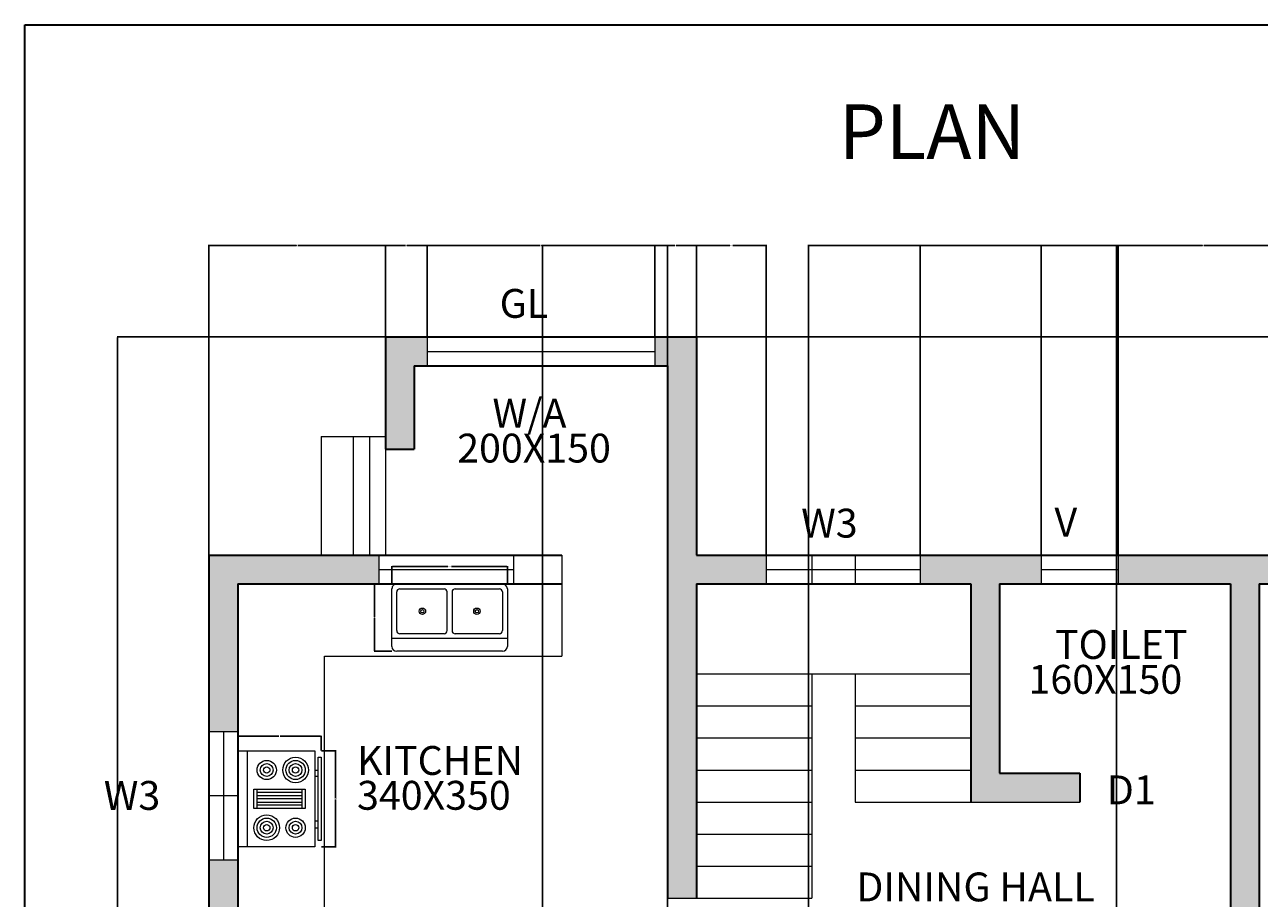
# Model space of a CAD drawing. Units: inches. Extents: x 1332 to 3175, y 1481 to 2088.
# Tile 3 of 5: x 1332 to 1717, y 1816 to 2088. Entities that reach past the tile are written whole.
import ezdxf

# ---------------------------------------------------------------- set-up
doc = ezdxf.new("R2010")
doc.units = ezdxf.units.IN
for name, color, linetype, lineweight in [('A-ANNO-DIMS', 2, 'Continuous', 18), ('A-ANNO-TEXT', 7, 'Continuous', 18), ('A-ANNO-TITL', 6, 'Continuous', 30), ('A-ANNO-TTLB', 7, 'Continuous', 35), ('A-AREA-IDEN', 7, 'Continuous', 18), ('A-EQPM', 8, 'Continuous', 18), ('A-FLOR-CASE', 8, 'Continuous', 18), ('A-FLOR-FIXT', 8, 'Continuous', 18), ('A-FLOR-STRS', 7, 'Continuous', 18), ('A-WALL', 7, 'Continuous', 35)]:
    doc.layers.add(name, color=color, linetype=linetype, lineweight=lineweight)
doc.layers.add('A-GLAZ', color=30, linetype='Continuous', lineweight=18, true_color=0xf8991e)
doc.layers.add('A-WALL-PATT', color=18, linetype='Continuous', lineweight=13, true_color=0x000000)
doc.styles.get("Standard").update_dxf_attribs({"font": 'arial.ttf'})
doc.dimstyles.get("Standard").update_dxf_attribs({"dimtxt": 0.18, "dimasz": 0.18, "dimexe": 0.18, "dimexo": 0.0625, "dimgap": 0.09, "dimtad": 0, "dimtih": 1, "dimtoh": 1, "dimdec": 4, "dimzin": 0, "dimdsep": 46, "dimtxsty": 'Standard', "dimcen": 0.09, "dimadec": 0, "dimazin": 0, "dimtfac": 1, "dimtdec": 4, "dimtofl": 0, "dimtmove": 0, "dimatfit": 3, "dimfxl": 1, "dimtolj": 1, "dimtzin": 0, "dimarcsym": 0})

# ---------------------------------------------------------------- blocks, each defined once
blk = doc.blocks.new('Range-Oven - 30 in top')
for p, q in [((0, -3), (30, -3)), ((12, -6), (18, -6)), ((13, -20), (13, -6)), ((14, -6), (14, -20)), ((15, -20), (15, -6)), ((16, -6), (16, -20)), ((17, -20), (17, -6)), ((18, -20), (12, -20)), ((6, -24), (6, -25)), ((8, -25), (8, -24)), ((22, -25), (22, -24)), ((24, -24), (24, -25))]:
    blk.add_line(p, q)
for points in [[(0, -24), (0, 0), (30, 0), (30, -24)], [(12, -21), (12, -5), (18, -5), (18, -21)], [(2, -26), (2, -25), (28, -25), (28, -26)]]:
    blk.add_lwpolyline(points, close=True)
for centre, radius in [((6, -9), 4), ((6, -9), 3), ((6, -9), 2), ((24, -9), 3), ((24, -9), 2), ((6, -9), 1), ((24, -9), 1), ((6, -18), 3), ((24, -18), 4), ((24, -18), 3), ((6, -18), 2), ((6, -18), 1), ((24, -18), 2), ((24, -18), 1)]:
    blk.add_circle(centre, radius)
blk = doc.blocks.new('Sink-double - 36 in top')
for p, q in [((-18, -4), (18, -4)), ((-0.75, -18.5), (-0.75, -6.5)), ((0.75, -6.5), (0.75, -18.5))]:
    blk.add_line(p, q)
for points in [[(-16.5, 0), (16.5, 0)], [(-18, -19.5), (-18, -1.5)], [(18, -1.5), (18, -19.5)], [(-16.5, -18.5), (-16.5, -6.5)], [(-15.5, -5.5), (-1.75, -5.5)], [(1.75, -5.5), (15.5, -5.5)], [(16.5, -6.5), (16.5, -18.5)], [(16.5, -21), (-16.5, -21)], [(-1.75, -19.5), (-15.5, -19.5)], [(15.5, -19.5), (1.75, -19.5)]]:
    blk.add_lwpolyline(points)
for centre, radius in [((-8.5, -12.5), 1), ((8.5, -12.5), 1), ((-8.5, -12.5), 0.5), ((8.5, -12.5), 0.5)]:
    blk.add_circle(centre, radius)
for centre, radius, start, end in [((-16.5, -1.5), 1.5, 90, 180), ((16.5, -1.5), 1.5, 0, 90), ((-15.5, -6.5), 1, 90, 180), ((-1.75, -6.5), 1, 0, 90), ((1.75, -6.5), 1, 90, 180), ((15.5, -6.5), 1, 0, 90), ((-15.5, -18.5), 1, 180, 270), ((-1.75, -18.5), 1, 270, 0), ((1.75, -18.5), 1, 180, 270), ((15.5, -18.5), 1, 270, 0), ((-16.5, -19.5), 1.5, 180, 270), ((16.5, -19.5), 1.5, 270, 0)]:
    blk.add_arc(centre, radius, start, end)
blk = doc.blocks.new('VENT-24')
for p, q in [((0, 9), (0, 0)), ((24, 9), (24, 0)), ((0, 4.5), (24, 4.5))]:
    blk.add_line(p, q)
blk = doc.blocks.new('*D27')
at = {"layer": 'A-ANNO-DIMS', "color": 0, "lineweight": -2, "transparency": 16777216}
for p, q in [((1424.69, 1862.12), (1429.31, 1862.12)), ((1429.13, 1861.94), (1429.13, 1847.3)), ((1429.13, 1832.3), (1429.13, 1846.94)), ((1424.69, 1832.12), (1429.31, 1832.12))]:
    blk.add_line(p, q, dxfattribs=at)
at = {"layer": 'A-ANNO-DIMS', "color": 0, "transparency": 16777216}
for points in [[(1429.1, 1861.94), (1429.16, 1861.94), (1429.13, 1862.12)], [(1429.1, 1832.3), (1429.16, 1832.3), (1429.13, 1832.12)]]:
    blk.add_solid(points, dxfattribs=at)
at = {"layer": 'Defpoints', "color": 0, "transparency": 16777216}
for p in [(1424.63, 1862.12), (1429.13, 1862.12), (1424.63, 1832.12)]:
    blk.add_point(p, dxfattribs=at)
at = {"layer": 'A-ANNO-DIMS', "color": 0, "transparency": 16777216, "insert": (1429.13, 1847.12), "char_height": 0.18, "attachment_point": 5}
blk.add_mtext('\\A1;RANGE 30', dxfattribs=at)
blk = doc.blocks.new('*D28')
at = {"layer": 'A-ANNO-DIMS', "color": 0, "lineweight": -2, "transparency": 16777216}
for p, q in [((1398.63, 1862.18), (1398.63, 1866.8)), ((1398.81, 1866.62), (1411.41, 1866.62)), ((1424.45, 1866.62), (1411.85, 1866.62)), ((1424.63, 1862.18), (1424.63, 1866.8))]:
    blk.add_line(p, q, dxfattribs=at)
at = {"layer": 'A-ANNO-DIMS', "color": 0, "transparency": 16777216}
for points in [[(1398.81, 1866.65), (1398.81, 1866.59), (1398.63, 1866.62)], [(1424.45, 1866.65), (1424.45, 1866.59), (1424.63, 1866.62)]]:
    blk.add_solid(points, dxfattribs=at)
at = {"layer": 'Defpoints', "color": 0, "transparency": 16777216}
for p in [(1398.63, 1866.62), (1398.63, 1862.12), (1424.63, 1862.12)]:
    blk.add_point(p, dxfattribs=at)
at = {"layer": 'A-ANNO-DIMS', "color": 0, "transparency": 16777216, "insert": (1411.63, 1866.62), "char_height": 0.18, "attachment_point": 5}
blk.add_mtext('\\A1;26', dxfattribs=at)
blk = doc.blocks.new('*D29')
at = {"layer": 'A-ANNO-DIMS', "color": 0, "lineweight": -2, "transparency": 16777216}
for p, q in [((1446.67, 1914.18), (1446.67, 1919.7)), ((1446.85, 1919.52), (1464.12, 1919.52)), ((1482.49, 1919.52), (1465.22, 1919.52)), ((1482.67, 1914.18), (1482.67, 1919.7))]:
    blk.add_line(p, q, dxfattribs=at)
at = {"layer": 'A-ANNO-DIMS', "color": 0, "transparency": 16777216}
for points in [[(1446.85, 1919.55), (1446.85, 1919.49), (1446.67, 1919.52)], [(1482.49, 1919.55), (1482.49, 1919.49), (1482.67, 1919.52)]]:
    blk.add_solid(points, dxfattribs=at)
at = {"layer": 'Defpoints', "color": 0, "transparency": 16777216}
for p in [(1446.67, 1919.52), (1446.67, 1914.12), (1482.67, 1914.12)]:
    blk.add_point(p, dxfattribs=at)
at = {"layer": 'A-ANNO-DIMS', "color": 0, "transparency": 16777216, "insert": (1464.67, 1919.52), "char_height": 0.18, "attachment_point": 5}
blk.add_mtext('\\A1;SINK 36', dxfattribs=at)
blk = doc.blocks.new('*D30')
at = {"layer": 'A-ANNO-DIMS', "color": 0, "lineweight": -2, "transparency": 16777216}
for p, q in [((1446.61, 1914.12), (1441.09, 1914.12)), ((1441.27, 1913.94), (1441.27, 1903.8)), ((1441.27, 1893.3), (1441.27, 1903.44)), ((1446.61, 1893.12), (1441.09, 1893.12))]:
    blk.add_line(p, q, dxfattribs=at)
at = {"layer": 'A-ANNO-DIMS', "color": 0, "transparency": 16777216}
for points in [[(1441.24, 1913.94), (1441.3, 1913.94), (1441.27, 1914.12)], [(1441.24, 1893.3), (1441.3, 1893.3), (1441.27, 1893.12)]]:
    blk.add_solid(points, dxfattribs=at)
at = {"layer": 'Defpoints', "color": 0, "transparency": 16777216}
for p in [(1446.67, 1914.12), (1441.27, 1893.12), (1446.67, 1893.12)]:
    blk.add_point(p, dxfattribs=at)
at = {"layer": 'A-ANNO-DIMS', "color": 0, "transparency": 16777216, "insert": (1441.27, 1903.62), "char_height": 0.18, "attachment_point": 5}
blk.add_mtext('\\A1;21', dxfattribs=at)
blk = doc.blocks.new('*D38')
at = {"layer": 'A-ANNO-DIMS', "color": 0, "lineweight": -2, "transparency": 16777216}
for p, q in [((1444.57, 1991.12), (1360.95, 1991.12)), ((1361.13, 1990.94), (1361.13, 1752.3)), ((1361.13, 1513.3), (1361.13, 1751.94)), ((1532.57, 1513.12), (1360.95, 1513.12))]:
    blk.add_line(p, q, dxfattribs=at)
at = {"layer": 'A-ANNO-DIMS', "color": 0, "transparency": 16777216}
for points in [[(1361.1, 1990.94), (1361.16, 1990.94), (1361.13, 1991.12)], [(1361.1, 1513.3), (1361.16, 1513.3), (1361.13, 1513.12)]]:
    blk.add_solid(points, dxfattribs=at)
at = {"layer": 'Defpoints', "color": 0, "transparency": 16777216}
for p in [(1361.13, 1991.12), (1444.63, 1991.12), (1532.63, 1513.12)]:
    blk.add_point(p, dxfattribs=at)
at = {"layer": 'A-ANNO-DIMS', "color": 0, "transparency": 16777216, "insert": (1361.13, 1752.12), "char_height": 0.18, "attachment_point": 5}
blk.add_mtext('\\A1;478', dxfattribs=at)
blk = doc.blocks.new('*D39')
at = {"layer": 'A-ANNO-DIMS', "color": 0, "lineweight": -2, "transparency": 16777216}
for p, q in [((1389.63, 1923.18), (1389.63, 2019.8)), ((1389.81, 2019.62), (1416.91, 2019.62)), ((1444.45, 2019.62), (1417.35, 2019.62)), ((1444.63, 1991.18), (1444.63, 2019.8))]:
    blk.add_line(p, q, dxfattribs=at)
at = {"layer": 'A-ANNO-DIMS', "color": 0, "transparency": 16777216}
for points in [[(1389.81, 2019.65), (1389.81, 2019.59), (1389.63, 2019.62)], [(1444.45, 2019.65), (1444.45, 2019.59), (1444.63, 2019.62)]]:
    blk.add_solid(points, dxfattribs=at)
at = {"layer": 'Defpoints', "color": 0, "transparency": 16777216}
for p in [(1444.63, 2019.62), (1444.63, 1991.12), (1389.63, 1923.12)]:
    blk.add_point(p, dxfattribs=at)
at = {"layer": 'A-ANNO-DIMS', "color": 0, "transparency": 16777216, "insert": (1417.13, 2019.62), "char_height": 0.18, "attachment_point": 5}
blk.add_mtext('\\A1;55', dxfattribs=at)
blk = doc.blocks.new('*D40')
at = {"layer": 'A-ANNO-DIMS', "color": 0, "lineweight": -2, "transparency": 16777216}
for p, q in [((1444.63, 1991.18), (1444.63, 2019.8)), ((1444.81, 2019.62), (1450.92, 2019.62)), ((1457.45, 2019.62), (1451.34, 2019.62)), ((1457.63, 1991.18), (1457.63, 2019.8))]:
    blk.add_line(p, q, dxfattribs=at)
at = {"layer": 'A-ANNO-DIMS', "color": 0, "transparency": 16777216}
for points in [[(1444.81, 2019.65), (1444.81, 2019.59), (1444.63, 2019.62)], [(1457.45, 2019.65), (1457.45, 2019.59), (1457.63, 2019.62)]]:
    blk.add_solid(points, dxfattribs=at)
at = {"layer": 'Defpoints', "color": 0, "transparency": 16777216}
for p in [(1457.63, 2019.62), (1444.63, 1991.12), (1457.63, 1991.12)]:
    blk.add_point(p, dxfattribs=at)
at = {"layer": 'A-ANNO-DIMS', "color": 0, "transparency": 16777216, "insert": (1451.13, 2019.62), "char_height": 0.18, "attachment_point": 5}
blk.add_mtext('\\A1;13', dxfattribs=at)
blk = doc.blocks.new('*D41')
at = {"layer": 'A-ANNO-DIMS', "color": 0, "lineweight": -2, "transparency": 16777216}
for p, q in [((1457.63, 1991.18), (1457.63, 2019.8)), ((1457.81, 2019.62), (1492.93, 2019.62)), ((1528.45, 2019.62), (1493.33, 2019.62)), ((1528.63, 1991.18), (1528.63, 2019.8))]:
    blk.add_line(p, q, dxfattribs=at)
at = {"layer": 'A-ANNO-DIMS', "color": 0, "transparency": 16777216}
for points in [[(1457.81, 2019.65), (1457.81, 2019.59), (1457.63, 2019.62)], [(1528.45, 2019.65), (1528.45, 2019.59), (1528.63, 2019.62)]]:
    blk.add_solid(points, dxfattribs=at)
at = {"layer": 'Defpoints', "color": 0, "transparency": 16777216}
for p in [(1528.63, 2019.62), (1457.63, 1991.12), (1528.63, 1991.12)]:
    blk.add_point(p, dxfattribs=at)
at = {"layer": 'A-ANNO-DIMS', "color": 0, "transparency": 16777216, "insert": (1493.13, 2019.62), "char_height": 0.18, "attachment_point": 5}
blk.add_mtext('\\A1;71', dxfattribs=at)
blk = doc.blocks.new('*D42')
at = {"layer": 'A-ANNO-DIMS', "color": 0, "lineweight": -2, "transparency": 16777216}
for p, q in [((1528.63, 1991.18), (1528.63, 2019.8)), ((1528.81, 2019.62), (1534.92, 2019.62)), ((1541.45, 2019.62), (1535.34, 2019.62)), ((1541.63, 1991.18), (1541.63, 2019.8))]:
    blk.add_line(p, q, dxfattribs=at)
at = {"layer": 'A-ANNO-DIMS', "color": 0, "transparency": 16777216}
for points in [[(1528.81, 2019.65), (1528.81, 2019.59), (1528.63, 2019.62)], [(1541.45, 2019.65), (1541.45, 2019.59), (1541.63, 2019.62)]]:
    blk.add_solid(points, dxfattribs=at)
at = {"layer": 'Defpoints', "color": 0, "transparency": 16777216}
for p in [(1541.63, 2019.62), (1528.63, 1991.12), (1541.63, 1991.12)]:
    blk.add_point(p, dxfattribs=at)
at = {"layer": 'A-ANNO-DIMS', "color": 0, "transparency": 16777216, "insert": (1535.13, 2019.62), "char_height": 0.18, "attachment_point": 5}
blk.add_mtext('\\A1;13', dxfattribs=at)
blk = doc.blocks.new('*D43')
at = {"layer": 'A-ANNO-DIMS', "color": 0, "lineweight": -2, "transparency": 16777216}
for p, q in [((1541.63, 1991.18), (1541.63, 2019.8)), ((1541.81, 2019.62), (1552.03, 2019.62)), ((1563.19, 2019.62), (1552.96, 2019.62)), ((1563.37, 1923.18), (1563.37, 2019.8))]:
    blk.add_line(p, q, dxfattribs=at)
at = {"layer": 'A-ANNO-DIMS', "color": 0, "transparency": 16777216}
for points in [[(1541.81, 2019.65), (1541.81, 2019.59), (1541.63, 2019.62)], [(1563.19, 2019.65), (1563.19, 2019.59), (1563.37, 2019.62)]]:
    blk.add_solid(points, dxfattribs=at)
at = {"layer": 'Defpoints', "color": 0, "transparency": 16777216}
for p in [(1563.37, 2019.62), (1541.63, 1991.12), (1563.37, 1923.12)]:
    blk.add_point(p, dxfattribs=at)
at = {"layer": 'A-ANNO-DIMS', "color": 0, "transparency": 16777216, "insert": (1552.5, 2019.62), "char_height": 0.18, "attachment_point": 5}
blk.add_mtext('\\A1;21.735', dxfattribs=at)
blk = doc.blocks.new('*D44')
at = {"layer": 'A-ANNO-DIMS', "color": 0, "lineweight": -2, "transparency": 16777216}
for p, q in [((1611.37, 1923.18), (1611.37, 2019.8)), ((1611.55, 2019.62), (1629.78, 2019.62)), ((1648.95, 2019.62), (1630.71, 2019.62)), ((1649.13, 1923.18), (1649.13, 2019.8))]:
    blk.add_line(p, q, dxfattribs=at)
at = {"layer": 'A-ANNO-DIMS', "color": 0, "transparency": 16777216}
for points in [[(1611.55, 2019.65), (1611.55, 2019.59), (1611.37, 2019.62)], [(1648.95, 2019.65), (1648.95, 2019.59), (1649.13, 2019.62)]]:
    blk.add_solid(points, dxfattribs=at)
at = {"layer": 'Defpoints', "color": 0, "transparency": 16777216}
for p in [(1649.13, 2019.62), (1611.37, 1923.12), (1649.13, 1923.12)]:
    blk.add_point(p, dxfattribs=at)
at = {"layer": 'A-ANNO-DIMS', "color": 0, "transparency": 16777216, "insert": (1630.25, 2019.62), "char_height": 0.18, "attachment_point": 5}
blk.add_mtext('\\A1;37.765', dxfattribs=at)
blk = doc.blocks.new('*D45')
at = {"layer": 'A-ANNO-DIMS', "color": 0, "lineweight": -2, "transparency": 16777216}
for p, q in [((1673.13, 1923.18), (1673.13, 2019.8)), ((1673.31, 2019.62), (1699.41, 2019.62)), ((1725.95, 2019.62), (1699.85, 2019.62)), ((1726.13, 1923.18), (1726.13, 2019.8))]:
    blk.add_line(p, q, dxfattribs=at)
at = {"layer": 'A-ANNO-DIMS', "color": 0, "transparency": 16777216}
for points in [[(1673.31, 2019.65), (1673.31, 2019.59), (1673.13, 2019.62)], [(1725.95, 2019.65), (1725.95, 2019.59), (1726.13, 2019.62)]]:
    blk.add_solid(points, dxfattribs=at)
at = {"layer": 'Defpoints', "color": 0, "transparency": 16777216}
for p in [(1726.13, 2019.62), (1673.13, 1923.12), (1726.13, 1923.12)]:
    blk.add_point(p, dxfattribs=at)
at = {"layer": 'A-ANNO-DIMS', "color": 0, "transparency": 16777216, "insert": (1699.63, 2019.62), "char_height": 0.18, "attachment_point": 5}
blk.add_mtext('\\A1;53', dxfattribs=at)
blk = doc.blocks.new('*D55')
at = {"layer": 'A-ANNO-DIMS', "color": 0, "lineweight": -2, "transparency": 16777216}
for p, q in [((1541.69, 1991.12), (1879.81, 1991.12)), ((1879.63, 1990.94), (1879.63, 1957.3)), ((1879.63, 1923.3), (1879.63, 1956.94)), ((1784.19, 1923.12), (1879.81, 1923.12))]:
    blk.add_line(p, q, dxfattribs=at)
at = {"layer": 'A-ANNO-DIMS', "color": 0, "transparency": 16777216}
for points in [[(1879.6, 1990.94), (1879.66, 1990.94), (1879.63, 1991.12)], [(1879.6, 1923.3), (1879.66, 1923.3), (1879.63, 1923.12)]]:
    blk.add_solid(points, dxfattribs=at)
at = {"layer": 'Defpoints', "color": 0, "transparency": 16777216}
for p in [(1541.63, 1991.12), (1879.63, 1991.12), (1784.13, 1923.12)]:
    blk.add_point(p, dxfattribs=at)
at = {"layer": 'A-ANNO-DIMS', "color": 0, "transparency": 16777216, "insert": (1879.63, 1957.12), "char_height": 0.18, "attachment_point": 5}
blk.add_mtext('\\A1;68', dxfattribs=at)
blk = doc.blocks.new('*D84')
at = {"layer": 'A-ANNO-DIMS', "color": 0, "lineweight": -2, "transparency": 16777216}
for p, q in [((1576.56, 1716.18), (1576.56, 2019.8)), ((1576.74, 2019.62), (1624.34, 2019.62)), ((1672.38, 2019.62), (1624.78, 2019.62)), ((1672.56, 1716.18), (1672.56, 2019.8))]:
    blk.add_line(p, q, dxfattribs=at)
at = {"layer": 'A-ANNO-DIMS', "color": 0, "transparency": 16777216}
for points in [[(1576.74, 2019.65), (1576.74, 2019.59), (1576.56, 2019.62)], [(1672.38, 2019.65), (1672.38, 2019.59), (1672.56, 2019.62)]]:
    blk.add_solid(points, dxfattribs=at)
at = {"layer": 'Defpoints', "color": 0, "transparency": 16777216}
for p in [(1672.56, 2019.62), (1576.56, 1716.12), (1672.56, 1716.12)]:
    blk.add_point(p, dxfattribs=at)
at = {"layer": 'A-ANNO-DIMS', "color": 0, "transparency": 16777216, "insert": (1624.56, 2019.62), "char_height": 0.18, "attachment_point": 5}
blk.add_mtext('\\A1;96', dxfattribs=at)
blk = doc.blocks.new('*D87')
at = {"layer": 'A-ANNO-DIMS', "color": 0, "lineweight": -2, "transparency": 16777216}
for p, q in [((1493.63, 1716.18), (1493.63, 2019.8)), ((1493.81, 2019.62), (1512.91, 2019.62)), ((1532.45, 2019.62), (1513.35, 2019.62)), ((1532.63, 1716.18), (1532.63, 2019.8))]:
    blk.add_line(p, q, dxfattribs=at)
at = {"layer": 'A-ANNO-DIMS', "color": 0, "transparency": 16777216}
for points in [[(1493.81, 2019.65), (1493.81, 2019.59), (1493.63, 2019.62)], [(1532.45, 2019.65), (1532.45, 2019.59), (1532.63, 2019.62)]]:
    blk.add_solid(points, dxfattribs=at)
at = {"layer": 'Defpoints', "color": 0, "transparency": 16777216}
for p in [(1532.63, 2019.62), (1493.63, 1716.12), (1532.63, 1716.12)]:
    blk.add_point(p, dxfattribs=at)
at = {"layer": 'A-ANNO-DIMS', "color": 0, "transparency": 16777216, "insert": (1513.13, 2019.62), "char_height": 0.18, "attachment_point": 5}
blk.add_mtext('\\A1;39', dxfattribs=at)

msp = doc.modelspace()

# ---------------------------------------------------------------- hatches: boundary and pattern name
at = {"layer": 'A-WALL-PATT'}
h = msp.add_hatch(color=256, dxfattribs=at)
h.dxf.hatch_style = 1
h.paths.add_polyline_path([(1398.6316, 1914.1183), (1442.6316, 1914.1183), (1442.6316, 1923.1183), (1389.6316, 1923.1183), (1389.6316, 1868.1183), (1398.6316, 1868.1183)])
h.paths.add_polyline_path([(1398.6316, 1828.1183), (1389.6316, 1828.1183), (1389.6316, 1759.1183), (1398.6316, 1759.1183), (1398.6316, 1771.1183), (1477.6316, 1771.1183), (1477.6316, 1716.1183), (1437.6316, 1716.1183), (1437.6316, 1707.1183), (1493.6316, 1707.1183), (1493.6316, 1716.1183), (1486.6316, 1716.1183), (1486.6316, 1771.1183), (1532.6316, 1771.1183), (1532.6316, 1780.1183), (1398.6316, 1780.1183)])
h.paths.add_polyline_path([(1398.6316, 1735.1183), (1389.6316, 1735.1183), (1389.6316, 1647.6183), (1398.6316, 1647.6183)])
h.paths.add_polyline_path([(1398.6316, 1599.6183), (1389.6316, 1599.6183), (1389.6316, 1533.1183), (1442.6316, 1533.1183), (1442.6316, 1542.1183), (1398.6316, 1542.1183)])
h.paths.add_polyline_path([(1541.6316, 1589.1183), (1576.5616, 1589.1183), (1576.5616, 1598.1183), (1541.6316, 1598.1183), (1541.6316, 1707.1183), (1576.5616, 1707.1183), (1576.5616, 1716.1183), (1532.6316, 1716.1183), (1532.6316, 1542.1183), (1490.6316, 1542.1183), (1490.6316, 1533.1183), (1541.6316, 1533.1183)])
h.paths.add_polyline_path([(1717.1316, 1707.1183), (1752.1316, 1707.1183), (1752.1316, 1716.1183), (1672.5616, 1716.1183), (1672.5616, 1707.1183), (1708.1316, 1707.1183), (1708.1316, 1598.1183), (1672.5616, 1598.1183), (1672.5616, 1589.1183), (1717.1316, 1589.1183)])
h.paths.add_polyline_path([(1851.1316, 1761.1183), (1842.1316, 1761.1183), (1842.1316, 1716.1183), (1800.1316, 1716.1183), (1800.1316, 1707.1183), (1851.1316, 1707.1183)])
h.paths.add_polyline_path([(1851.1316, 1855.1183), (1784.1316, 1855.1183), (1784.1316, 1923.1183), (1750.1316, 1923.1183), (1750.1316, 1914.1183), (1775.1316, 1914.1183), (1775.1316, 1855.1183), (1750.1316, 1855.1183), (1750.1316, 1846.1183), (1842.1316, 1846.1183), (1842.1316, 1801.1183), (1851.1316, 1801.1183)])
h.paths.add_polyline_path([(1717.1316, 1914.1183), (1726.1316, 1914.1183), (1726.1316, 1923.1183), (1673.1316, 1923.1183), (1673.1316, 1914.1183), (1708.1316, 1914.1183), (1708.1316, 1755.1183), (1717.1316, 1755.1183)])
h.paths.add_polyline_path([(1661.1316, 1855.1183), (1636.1316, 1855.1183), (1636.1316, 1914.1183), (1649.1316, 1914.1183), (1649.1316, 1923.1183), (1611.3665, 1923.1183), (1611.3665, 1914.1183), (1627.1316, 1914.1183), (1627.1316, 1846.1183), (1661.1316, 1846.1183)])
h.paths.add_polyline_path([(1541.6316, 1914.1183), (1563.3665, 1914.1183), (1563.3665, 1923.1183), (1541.6316, 1923.1183), (1541.6316, 1991.1183), (1528.6316, 1991.1183), (1528.6316, 1982.1183), (1532.6316, 1982.1183), (1532.6316, 1914.1183), (1532.6316, 1816.1183), (1541.6316, 1816.1183)])
h.paths.add_polyline_path([(1453.6316, 1982.1183), (1457.6316, 1982.1183), (1457.6316, 1991.1183), (1444.6316, 1991.1183), (1444.6316, 1956.1183), (1453.6316, 1956.1183)])

# ---------------------------------------------------------------- linework, layer by layer
at = {"layer": 'A-ANNO-TTLB'}
msp.add_lwpolyline([(1332.1674, 2088.4777), (3159.6908, 2088.4777), (3159.6908, 1485.6439), (1332.1674, 1485.6439)], close=True, dxfattribs=at)
at = {"layer": 'A-FLOR-CASE'}
for p, q in [((1499.6316, 1923.1183), (1499.6316, 1891.601)), ((1425.7005, 1891.601), (1499.6316, 1891.601)), ((1425.7005, 1780.1183), (1425.7005, 1891.601))]:
    msp.add_line(p, q, dxfattribs=at)
at = {"layer": 'A-FLOR-STRS'}
for p, q in [((1424.6316, 1960.1183), (1444.6316, 1960.1183)), ((1424.6316, 1960.1183), (1424.6316, 1923.1183)), ((1434.6316, 1960.1183), (1434.6316, 1923.1183)), ((1439.6316, 1960.1183), (1439.6316, 1923.1183)), ((1444.6316, 1960.1183), (1444.6316, 1923.1183)), ((1541.6316, 1886.1183), (1577.6316, 1886.1183)), ((1577.6316, 1886.1183), (1627.1316, 1886.1183)), ((1577.6316, 1886.1183), (1577.6316, 1816.1183)), ((1591.1316, 1886.1183), (1591.1316, 1846.1183)), ((1541.6316, 1876.1183), (1577.6316, 1876.1183)), ((1591.1316, 1876.1183), (1627.1316, 1876.1183)), ((1541.6316, 1866.1183), (1577.6316, 1866.1183)), ((1591.1316, 1866.1183), (1627.1316, 1866.1183)), ((1541.6316, 1856.1183), (1577.6316, 1856.1183)), ((1591.1316, 1856.1183), (1627.1316, 1856.1183)), ((1541.6316, 1846.1183), (1577.6316, 1846.1183)), ((1591.1316, 1846.1183), (1661.1316, 1846.1183)), ((1541.6316, 1836.1183), (1577.6316, 1836.1183)), ((1541.6316, 1826.1183), (1577.6316, 1826.1183)), ((1532.6316, 1816.1183), (1577.6316, 1816.1183))]:
    msp.add_line(p, q, dxfattribs=at)
at = {"layer": 'A-GLAZ'}
for p, q in [((1457.6316, 1991.1183), (1457.6316, 1982.1183)), ((1528.6316, 1991.1183), (1528.6316, 1982.1183)), ((1457.6316, 1986.6183), (1528.6316, 1986.6183)), ((1442.6316, 1923.1183), (1442.6316, 1914.1183)), ((1484.6316, 1923.1183), (1484.6316, 1914.1183)), ((1563.3665, 1923.1183), (1563.3665, 1914.1183)), ((1563.3665, 1923.1183), (1563.3665, 1914.1183)), ((1577.6316, 1923.1183), (1577.6316, 1914.1183)), ((1591.1316, 1923.1183), (1591.1316, 1914.1183)), ((1611.3665, 1923.1183), (1611.3665, 1914.1183)), ((1442.6316, 1918.6183), (1484.6316, 1918.6183)), ((1563.3665, 1918.6183), (1611.3665, 1918.6183)), ((1389.6316, 1868.1183), (1398.6316, 1868.1183)), ((1394.1316, 1868.1183), (1394.1316, 1828.1183)), ((1389.6316, 1848.1183), (1398.6316, 1848.1183)), ((1389.6316, 1828.1183), (1398.6316, 1828.1183))]:
    msp.add_line(p, q, dxfattribs=at)
at = {"layer": 'A-WALL'}
for p, q in [((1444.6316, 1991.1183), (1444.6316, 1956.1183)), ((1444.6316, 1991.1183), (1541.6316, 1991.1183)), ((1541.6316, 1991.1183), (1541.6316, 1923.1183)), ((1453.6316, 1982.1183), (1453.6316, 1956.1183)), ((1453.6316, 1982.1183), (1532.6316, 1982.1183)), ((1532.6316, 1982.1183), (1532.6316, 1914.1183)), ((1444.6316, 1956.1183), (1453.6316, 1956.1183)), ((1532.6316, 1927.1183), (1532.6316, 1923.1183)), ((1389.6316, 1923.1183), (1499.6316, 1923.1183)), ((1389.6316, 1923.1183), (1389.6316, 1533.1183)), ((1541.6316, 1923.1183), (1784.1316, 1923.1183)), ((1398.6316, 1914.1183), (1499.6316, 1914.1183)), ((1398.6316, 1914.1183), (1398.6316, 1780.1183)), ((1532.6316, 1914.1183), (1532.6316, 1816.1183)), ((1532.6316, 1914.1183), (1532.6316, 1816.1183)), ((1541.6316, 1914.1183), (1541.6316, 1816.1183)), ((1541.6316, 1914.1183), (1627.1316, 1914.1183)), ((1627.1316, 1914.1183), (1627.1316, 1846.1183)), ((1636.1316, 1914.1183), (1636.1316, 1855.1183)), ((1636.1316, 1914.1183), (1708.1316, 1914.1183)), ((1708.1316, 1914.1183), (1708.1316, 1755.1183)), ((1717.1316, 1914.1183), (1717.1316, 1755.1183)), ((1717.1316, 1914.1183), (1775.1316, 1914.1183)), ((1636.1316, 1855.1183), (1661.1316, 1855.1183)), ((1661.1316, 1855.1183), (1661.1316, 1846.1183))]:
    msp.add_line(p, q, dxfattribs=at)

# ---------------------------------------------------------------- block references
at = {"layer": 'A-EQPM', "rotation": 90}
msp.add_blockref('Range-Oven - 30 in top', (1398.6316, 1832.1183), dxfattribs=at)
at = {"layer": 'A-FLOR-FIXT', "rotation": 180}
msp.add_blockref('Sink-double - 36 in top', (1464.6705, 1893.1183), dxfattribs=at)
at = {"layer": 'A-GLAZ'}
msp.add_blockref('VENT-24', (1649.1316, 1914.1183), dxfattribs=at)

# ---------------------------------------------------------------- texts
at = {"layer": 'A-ANNO-TEXT'}
for s, p in [('    GL', (1469.2651, 1997.0846)), ('    W3', (1563.289, 1928.5764)), ('      V', (1636.7657, 1928.8639)), ('    W3', (1345.8302, 1843.6895)), ('      D1', (1653.0711, 1845.4202))]:
    msp.add_text(s, height=9, dxfattribs=at).set_placement(p)
at = {"layer": 'A-ANNO-TITL'}
msp.add_text('   PLAN', height=17, dxfattribs=at).set_placement((1570.4287, 2046.6351))
at = {"layer": 'A-AREA-IDEN'}
for s, p in [('    W/A', (1467.0304, 1962.8399)), ('200X150', (1467.0304, 1951.9753)), ('   TOILET', (1645.1737, 1890.747)), ('160X150', (1645.1737, 1879.8824)), ('KITCHEN', (1435.7969, 1854.5916)), ('340X350', (1435.7969, 1843.727)), ('DINING HALL', (1591.4784, 1815.1673))]:
    msp.add_text(s, height=9, dxfattribs=at).set_placement(p)

# ---------------------------------------------------------------- dimensions: what is measured, and where the dimension line sits
at = {"layer": 'A-ANNO-DIMS'}
for base, p1, p2, override, picture, middle in [((1444.6316, 2019.6183), (1389.6316, 1923.1183), (1444.6316, 1991.1183), {"dimdec": 0, "dimlfac": 1, "dimrnd": 0, "dimzin": 0, "dimdsep": 46, "dimlunit": 2}, '*D39', (1417.1316, 2019.6183)), ((1457.6316, 2019.6183), (1444.6316, 1991.1183), (1457.6316, 1991.1183), {"dimdec": 0, "dimlfac": 1, "dimrnd": 0, "dimzin": 0, "dimdsep": 46, "dimlunit": 2}, '*D40', (1451.1316, 2019.6183)), ((1528.6316, 2019.6183), (1457.6316, 1991.1183), (1528.6316, 1991.1183), {"dimdec": 0, "dimlfac": 1, "dimrnd": 0, "dimzin": 0, "dimdsep": 46, "dimlunit": 2}, '*D41', (1493.1316, 2019.6183)), ((1532.6316, 2019.6183), (1493.6316, 1716.1183), (1532.6316, 1716.1183), {"dimdec": 0, "dimlfac": 1, "dimrnd": 0, "dimzin": 0, "dimdsep": 46, "dimlunit": 2}, '*D87', (1513.1316, 2019.6183)), ((1541.6316, 2019.6183), (1528.6316, 1991.1183), (1541.6316, 1991.1183), {"dimdec": 0, "dimlfac": 1, "dimrnd": 0, "dimzin": 0, "dimdsep": 46, "dimlunit": 2}, '*D42', (1535.1316, 2019.6183)), ((1563.3665, 2019.6183), (1541.6316, 1991.1183), (1563.3665, 1923.1183), {"dimdec": 3, "dimlfac": 1, "dimrnd": 0, "dimzin": 0, "dimdsep": 46, "dimlunit": 2}, '*D43', (1552.499, 2019.6183)), ((1672.5616, 2019.6183), (1576.5616, 1716.1183), (1672.5616, 1716.1183), {"dimdec": 0, "dimlfac": 1, "dimrnd": 0, "dimzin": 0, "dimdsep": 46, "dimlunit": 2}, '*D84', (1624.5616, 2019.6183)), ((1649.1316, 2019.6183), (1611.3665, 1923.1183), (1649.1316, 1923.1183), {"dimdec": 3, "dimlfac": 1, "dimrnd": 0, "dimzin": 0, "dimdsep": 46, "dimlunit": 2}, '*D44', (1630.249, 2019.6183)), ((1726.1316, 2019.6183), (1673.1316, 1923.1183), (1726.1316, 1923.1183), {"dimdec": 0, "dimlfac": 1, "dimrnd": 0, "dimzin": 0, "dimdsep": 46, "dimlunit": 2}, '*D45', (1699.6316, 2019.6183))]:
    dim = msp.add_linear_dim(base=base, p1=p1, p2=p2, dimstyle='Standard', override=override, dxfattribs=at)
    dim.commit()
    dim.dimension.update_dxf_attribs({"geometry": picture, "text_midpoint": middle})
for base, p1, p2, angle, picture, middle in [((1361.1316, 1991.1183), (1532.6316, 1513.1183), (1444.6316, 1991.1183), 90, '*D38', (1361.1316, 1752.1183)), ((1879.6316, 1991.1183), (1784.1316, 1923.1183), (1541.6316, 1991.1183), 90, '*D55', (1879.6316, 1957.1183)), ((1441.2705, 1893.1183), (1446.6705, 1914.1183), (1446.6705, 1893.1183), 270, '*D30', (1441.2705, 1903.6183)), ((1398.6316, 1866.6183), (1424.6316, 1862.1183), (1398.6316, 1862.1183), 180, '*D28', (1411.6316, 1866.6183))]:
    dim = msp.add_linear_dim(base=base, p1=p1, p2=p2, angle=angle, dimstyle='Standard', override={"dimdec": 0, "dimlfac": 1, "dimrnd": 0, "dimzin": 0, "dimdsep": 46, "dimlunit": 2}, dxfattribs=at)
    dim.commit()
    dim.dimension.update_dxf_attribs({"geometry": picture, "text_midpoint": middle})
for base, p1, p2, angle, text, picture, middle in [((1446.6705, 1919.5183), (1482.6705, 1914.1183), (1446.6705, 1914.1183), 180, 'SINK <>', '*D29', (1464.6705, 1919.5183)), ((1429.1316, 1862.1183), (1424.6316, 1832.1183), (1424.6316, 1862.1183), 90, 'RANGE <>', '*D27', (1429.1316, 1847.1183))]:
    dim = msp.add_linear_dim(base=base, p1=p1, p2=p2, angle=angle, text=text, dimstyle='Standard', override={"dimdec": 0, "dimlfac": 1, "dimrnd": 0, "dimzin": 0, "dimdsep": 46, "dimlunit": 2}, dxfattribs=at)
    dim.commit()
    dim.dimension.update_dxf_attribs({"geometry": picture, "text_midpoint": middle})

doc.saveas('drawing.dxf')
